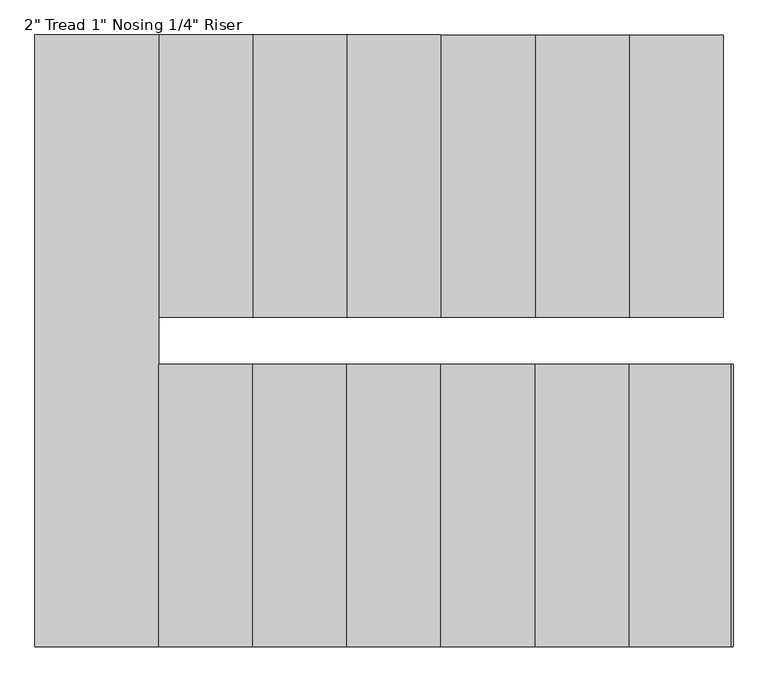
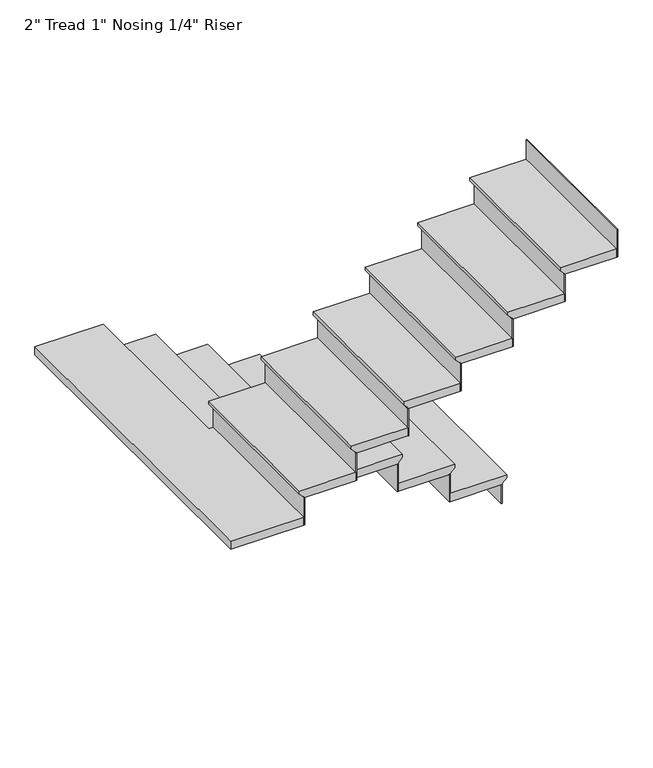
"""IFC4 building model written with IfcOpenShell, lengths in millimetres: stair flight geometry."""

from ifc_helpers import new_model, si_unit, origin, place, context, project, spatial, faceted_brep, source, transform, mapped, element, save


def stair_flight_2ee17b95(model_context):
    return source(origin(), model_context, "Body", "Brep", [
        faceted_brep([(3727.9146873, 3708.4, 3198.2833333), (3727.9146873, 3708.4, 3217.3333333), (3727.9146873, 2794.0, 3217.3333333), (3727.9146873, 2794.0, 3198.2833333), (3702.5146873, 3708.4, 3172.8833333), (3702.5146873, 2794.0, 3172.8833333), (3397.7146873, 3708.4, 3217.3333333), (3397.7146873, 2794.0, 3217.3333333), (3702.5146873, 2794.0, 3166.5333333), (3397.7146873, 2794.0, 3166.5333333), (3397.7146873, 3708.4, 3166.5333333), (3702.5146873, 3708.4, 3166.5333333)], [[[0, 1, 2, 3]], [[4, 0, 3, 5]], [[2, 1, 6, 7]], [[8, 9, 10, 11]], [[2, 7, 9, 8, 5, 3]], [[8, 11, 4, 5]], [[6, 1, 0, 4, 11, 10]], [[7, 6, 10, 9]]]),
        faceted_brep([(3702.5146873, 3708.4, 3166.5333333), (3702.5146873, 3708.4, 3048.0), (3696.1646873, 3708.4, 3048.0), (3696.1646873, 3708.4, 3166.5333333), (3702.5146873, 2794.0, 3166.5333333), (3696.1646873, 2794.0, 3166.5333333), (3696.1646873, 2794.0, 3048.0), (3702.5146873, 2794.0, 3048.0)], [[[0, 1, 2, 3]], [[4, 5, 6, 7]], [[1, 0, 4, 7]], [[2, 1, 7, 6]], [[3, 2, 6, 5]], [[0, 3, 5, 4]]]),
        faceted_brep([(3397.7146873, 3708.4, 3335.8666667), (3397.7146873, 3708.4, 3166.5333333), (3391.3646873, 3708.4, 3166.5333333), (3391.3646873, 3708.4, 3335.8666667), (3397.7146873, 2794.0, 3335.8666667), (3391.3646873, 2794.0, 3335.8666667), (3391.3646873, 2794.0, 3166.5333333), (3397.7146873, 2794.0, 3166.5333333)], [[[0, 1, 2, 3]], [[4, 5, 6, 7]], [[1, 0, 4, 7]], [[2, 1, 7, 6]], [[3, 2, 6, 5]], [[0, 3, 5, 4]]]),
        faceted_brep([(3423.1146873, 2794.0, 3386.6666667), (3423.1146873, 3708.4, 3386.6666667), (3092.9146873, 3708.4, 3386.6666667), (3092.9146873, 2794.0, 3386.6666667), (3397.7146873, 2794.0, 3335.8666667), (3092.9146873, 2794.0, 3335.8666667), (3092.9146873, 3708.4, 3335.8666667), (3397.7146873, 3708.4, 3335.8666667), (3397.7146873, 2794.0, 3342.2166667), (3423.1146873, 2794.0, 3367.6166667), (3397.7146873, 3708.4, 3342.2166667), (3423.1146873, 3708.4, 3367.6166667)], [[[0, 1, 2, 3]], [[4, 5, 6, 7]], [[0, 3, 5, 4, 8, 9]], [[4, 7, 10, 8]], [[2, 1, 11, 10, 7, 6]], [[3, 2, 6, 5]], [[11, 1, 0, 9]], [[10, 11, 9, 8]]]),
        faceted_brep([(3092.9146873, 3708.4, 3505.2), (3092.9146873, 3708.4, 3335.8666667), (3086.5646873, 3708.4, 3335.8666667), (3086.5646873, 3708.4, 3505.2), (3092.9146873, 2794.0, 3505.2), (3086.5646873, 2794.0, 3505.2), (3086.5646873, 2794.0, 3335.8666667), (3092.9146873, 2794.0, 3335.8666667)], [[[0, 1, 2, 3]], [[4, 5, 6, 7]], [[1, 0, 4, 7]], [[2, 1, 7, 6]], [[3, 2, 6, 5]], [[0, 3, 5, 4]]]),
        faceted_brep([(3118.3146873, 2794.0, 3556.0), (3118.3146873, 3708.4, 3556.0), (2788.1146873, 3708.4, 3556.0), (2788.1146873, 2794.0, 3556.0), (3092.9146873, 2794.0, 3505.2), (2788.1146873, 2794.0, 3505.2), (2788.1146873, 3708.4, 3505.2), (3092.9146873, 3708.4, 3505.2), (3092.9146873, 2794.0, 3511.55), (3118.3146873, 2794.0, 3536.95), (3092.9146873, 3708.4, 3511.55), (3118.3146873, 3708.4, 3536.95)], [[[0, 1, 2, 3]], [[4, 5, 6, 7]], [[0, 3, 5, 4, 8, 9]], [[4, 7, 10, 8]], [[2, 1, 11, 10, 7, 6]], [[3, 2, 6, 5]], [[11, 1, 0, 9]], [[10, 11, 9, 8]]]),
        faceted_brep([(2788.1146873, 3708.4, 3674.5333333), (2788.1146873, 3708.4, 3505.2), (2781.7646873, 3708.4, 3505.2), (2781.7646873, 3708.4, 3674.5333333), (2788.1146873, 2794.0, 3674.5333333), (2781.7646873, 2794.0, 3674.5333333), (2781.7646873, 2794.0, 3505.2), (2788.1146873, 2794.0, 3505.2)], [[[0, 1, 2, 3]], [[4, 5, 6, 7]], [[1, 0, 4, 7]], [[2, 1, 7, 6]], [[3, 2, 6, 5]], [[0, 3, 5, 4]]]),
        faceted_brep([(2813.5146873, 2794.0, 3725.3333333), (2813.5146873, 3708.4, 3725.3333333), (2483.3146873, 3708.4, 3725.3333333), (2483.3146873, 2794.0, 3725.3333333), (2788.1146873, 2794.0, 3674.5333333), (2483.3146873, 2794.0, 3674.5333333), (2483.3146873, 3708.4, 3674.5333333), (2788.1146873, 3708.4, 3674.5333333), (2788.1146873, 2794.0, 3680.8833333), (2813.5146873, 2794.0, 3706.2833333), (2788.1146873, 3708.4, 3680.8833333), (2813.5146873, 3708.4, 3706.2833333)], [[[0, 1, 2, 3]], [[4, 5, 6, 7]], [[0, 3, 5, 4, 8, 9]], [[4, 7, 10, 8]], [[2, 1, 11, 10, 7, 6]], [[3, 2, 6, 5]], [[11, 1, 0, 9]], [[10, 11, 9, 8]]]),
        faceted_brep([(2483.3146873, 3708.4, 3843.8666667), (2483.3146873, 3708.4, 3674.5333333), (2476.9646873, 3708.4, 3674.5333333), (2476.9646873, 3708.4, 3843.8666667), (2483.3146873, 2794.0, 3843.8666667), (2476.9646873, 2794.0, 3843.8666667), (2476.9646873, 2794.0, 3674.5333333), (2483.3146873, 2794.0, 3674.5333333)], [[[0, 1, 2, 3]], [[4, 5, 6, 7]], [[1, 0, 4, 7]], [[2, 1, 7, 6]], [[3, 2, 6, 5]], [[0, 3, 5, 4]]]),
        faceted_brep([(2508.7146873, 2794.0, 3894.6666667), (2508.7146873, 3708.4, 3894.6666667), (2178.5146873, 3708.4, 3894.6666667), (2178.5146873, 2794.0, 3894.6666667), (2483.3146873, 2794.0, 3843.8666667), (2178.5146873, 2794.0, 3843.8666667), (2178.5146873, 3708.4, 3843.8666667), (2483.3146873, 3708.4, 3843.8666667), (2483.3146873, 2794.0, 3850.2166667), (2508.7146873, 2794.0, 3875.6166667), (2483.3146873, 3708.4, 3850.2166667), (2508.7146873, 3708.4, 3875.6166667)], [[[0, 1, 2, 3]], [[4, 5, 6, 7]], [[0, 3, 5, 4, 8, 9]], [[4, 7, 10, 8]], [[2, 1, 11, 10, 7, 6]], [[3, 2, 6, 5]], [[11, 1, 0, 9]], [[10, 11, 9, 8]]]),
        faceted_brep([(2178.5146873, 3708.4, 4013.2), (2178.5146873, 3708.4, 3843.8666667), (2172.1646873, 3708.4, 3843.8666667), (2172.1646873, 3708.4, 4013.2), (2178.5146873, 2794.0, 4013.2), (2172.1646873, 2794.0, 4013.2), (2172.1646873, 2794.0, 3843.8666667), (2178.5146873, 2794.0, 3843.8666667)], [[[0, 1, 2, 3]], [[4, 5, 6, 7]], [[1, 0, 4, 7]], [[2, 1, 7, 6]], [[3, 2, 6, 5]], [[0, 3, 5, 4]]]),
        faceted_brep([(2203.9146873, 2794.0, 4064.0), (2203.9146873, 3708.4, 4064.0), (1873.7146873, 3708.4, 4064.0), (1873.7146873, 2794.0, 4064.0), (2178.5146873, 2794.0, 4013.2), (1873.7146873, 2794.0, 4013.2), (1873.7146873, 3708.4, 4013.2), (2178.5146873, 3708.4, 4013.2), (2178.5146873, 2794.0, 4019.55), (2203.9146873, 2794.0, 4044.95), (2178.5146873, 3708.4, 4019.55), (2203.9146873, 3708.4, 4044.95)], [[[0, 1, 2, 3]], [[4, 5, 6, 7]], [[0, 3, 5, 4, 8, 9]], [[4, 7, 10, 8]], [[2, 1, 11, 10, 7, 6]], [[3, 2, 6, 5]], [[11, 1, 0, 9]], [[10, 11, 9, 8]]]),
        faceted_brep([(1873.7146873, 3708.4, 4182.5333333), (1873.7146873, 3708.4, 4013.2), (1867.3646873, 3708.4, 4013.2), (1867.3646873, 3708.4, 4182.5333333), (1873.7146873, 2794.0, 4182.5333333), (1867.3646873, 2794.0, 4182.5333333), (1867.3646873, 2794.0, 4013.2), (1873.7146873, 2794.0, 4013.2)], [[[0, 1, 2, 3]], [[4, 5, 6, 7]], [[1, 0, 4, 7]], [[2, 1, 7, 6]], [[3, 2, 6, 5]], [[0, 3, 5, 4]]]),
        faceted_brep([(1924.5146873, 2641.6, 4233.3333333), (1899.1146873, 2641.6, 4233.3333333), (1899.1146873, 3708.4, 4233.3333333), (1498.6, 3708.4, 4233.3333333), (1498.6, 1727.2, 4233.3333333), (1924.5146873, 1727.2, 4233.3333333), (1899.1146873, 2641.6, 4182.5333333), (1924.5146873, 2641.6, 4182.5333333), (1924.5146873, 1727.2, 4182.5333333), (1498.6, 1727.2, 4182.5333333), (1498.6, 3708.4, 4182.5333333), (1873.7146873, 3708.4, 4182.5333333), (1873.7146873, 2794.0, 4182.5333333), (1899.1146873, 2794.0, 4182.5333333), (1899.1146873, 2794.0, 4214.2833333), (1899.1146873, 3708.4, 4214.2833333), (1873.7146873, 2794.0, 4188.8833333), (1873.7146873, 3708.4, 4188.8833333)], [[[0, 1, 2, 3, 4, 5]], [[6, 7, 8, 9, 10, 11, 12, 13]], [[1, 0, 7, 6]], [[2, 1, 6, 13, 14, 15]], [[13, 12, 16, 14]], [[12, 11, 17, 16]], [[3, 2, 15, 17, 11, 10]], [[4, 3, 10, 9]], [[5, 4, 9, 8]], [[0, 5, 8, 7]], [[17, 15, 14, 16]]]),
        faceted_brep([(1924.5146873, 1727.2, 4351.8666667), (1924.5146873, 1727.2, 4182.5333333), (1930.8646873, 1727.2, 4182.5333333), (1930.8646873, 1727.2, 4351.8666667), (1924.5146873, 2641.6, 4351.8666667), (1930.8646873, 2641.6, 4351.8666667), (1930.8646873, 2641.6, 4182.5333333), (1924.5146873, 2641.6, 4182.5333333)], [[[0, 1, 2, 3]], [[4, 5, 6, 7]], [[1, 0, 4, 7]], [[2, 1, 7, 6]], [[3, 2, 6, 5]], [[0, 3, 5, 4]]]),
        faceted_brep([(1899.1146873, 2641.6, 4402.6666667), (1899.1146873, 1727.2, 4402.6666667), (2229.3146873, 1727.2, 4402.6666667), (2229.3146873, 2641.6, 4402.6666667), (1924.5146873, 2641.6, 4351.8666667), (2229.3146873, 2641.6, 4351.8666667), (2229.3146873, 1727.2, 4351.8666667), (1924.5146873, 1727.2, 4351.8666667), (1924.5146873, 2641.6, 4358.2166667), (1899.1146873, 2641.6, 4383.6166667), (1924.5146873, 1727.2, 4358.2166667), (1899.1146873, 1727.2, 4383.6166667)], [[[0, 1, 2, 3]], [[4, 5, 6, 7]], [[0, 3, 5, 4, 8, 9]], [[4, 7, 10, 8]], [[2, 1, 11, 10, 7, 6]], [[3, 2, 6, 5]], [[11, 1, 0, 9]], [[10, 11, 9, 8]]]),
        faceted_brep([(2229.3146873, 1727.2, 4521.2), (2229.3146873, 1727.2, 4351.8666667), (2235.6646873, 1727.2, 4351.8666667), (2235.6646873, 1727.2, 4521.2), (2229.3146873, 2641.6, 4521.2), (2235.6646873, 2641.6, 4521.2), (2235.6646873, 2641.6, 4351.8666667), (2229.3146873, 2641.6, 4351.8666667)], [[[0, 1, 2, 3]], [[4, 5, 6, 7]], [[1, 0, 4, 7]], [[2, 1, 7, 6]], [[3, 2, 6, 5]], [[0, 3, 5, 4]]]),
        faceted_brep([(2203.9146873, 2641.6, 4572.0), (2203.9146873, 1727.2, 4572.0), (2534.1146873, 1727.2, 4572.0), (2534.1146873, 2641.6, 4572.0), (2229.3146873, 2641.6, 4521.2), (2534.1146873, 2641.6, 4521.2), (2534.1146873, 1727.2, 4521.2), (2229.3146873, 1727.2, 4521.2), (2229.3146873, 2641.6, 4527.55), (2203.9146873, 2641.6, 4552.95), (2229.3146873, 1727.2, 4527.55), (2203.9146873, 1727.2, 4552.95)], [[[0, 1, 2, 3]], [[4, 5, 6, 7]], [[0, 3, 5, 4, 8, 9]], [[4, 7, 10, 8]], [[2, 1, 11, 10, 7, 6]], [[3, 2, 6, 5]], [[11, 1, 0, 9]], [[10, 11, 9, 8]]]),
        faceted_brep([(2534.1146873, 1727.2, 4690.5333333), (2534.1146873, 1727.2, 4521.2), (2540.4646873, 1727.2, 4521.2), (2540.4646873, 1727.2, 4690.5333333), (2534.1146873, 2641.6, 4690.5333333), (2540.4646873, 2641.6, 4690.5333333), (2540.4646873, 2641.6, 4521.2), (2534.1146873, 2641.6, 4521.2)], [[[0, 1, 2, 3]], [[4, 5, 6, 7]], [[1, 0, 4, 7]], [[2, 1, 7, 6]], [[3, 2, 6, 5]], [[0, 3, 5, 4]]]),
        faceted_brep([(2508.7146873, 2641.6, 4741.3333333), (2508.7146873, 1727.2, 4741.3333333), (2838.9146873, 1727.2, 4741.3333333), (2838.9146873, 2641.6, 4741.3333333), (2534.1146873, 2641.6, 4690.5333333), (2838.9146873, 2641.6, 4690.5333333), (2838.9146873, 1727.2, 4690.5333333), (2534.1146873, 1727.2, 4690.5333333), (2534.1146873, 2641.6, 4696.8833333), (2508.7146873, 2641.6, 4722.2833333), (2534.1146873, 1727.2, 4696.8833333), (2508.7146873, 1727.2, 4722.2833333)], [[[0, 1, 2, 3]], [[4, 5, 6, 7]], [[0, 3, 5, 4, 8, 9]], [[4, 7, 10, 8]], [[2, 1, 11, 10, 7, 6]], [[3, 2, 6, 5]], [[11, 1, 0, 9]], [[10, 11, 9, 8]]]),
        faceted_brep([(2838.9146873, 1727.2, 4859.8666667), (2838.9146873, 1727.2, 4690.5333333), (2845.2646873, 1727.2, 4690.5333333), (2845.2646873, 1727.2, 4859.8666667), (2838.9146873, 2641.6, 4859.8666667), (2845.2646873, 2641.6, 4859.8666667), (2845.2646873, 2641.6, 4690.5333333), (2838.9146873, 2641.6, 4690.5333333)], [[[0, 1, 2, 3]], [[4, 5, 6, 7]], [[1, 0, 4, 7]], [[2, 1, 7, 6]], [[3, 2, 6, 5]], [[0, 3, 5, 4]]]),
        faceted_brep([(2813.5146873, 2641.6, 4910.6666667), (2813.5146873, 1727.2, 4910.6666667), (3143.7146873, 1727.2, 4910.6666667), (3143.7146873, 2641.6, 4910.6666667), (2838.9146873, 2641.6, 4859.8666667), (3143.7146873, 2641.6, 4859.8666667), (3143.7146873, 1727.2, 4859.8666667), (2838.9146873, 1727.2, 4859.8666667), (2838.9146873, 2641.6, 4866.2166667), (2813.5146873, 2641.6, 4891.6166667), (2838.9146873, 1727.2, 4866.2166667), (2813.5146873, 1727.2, 4891.6166667)], [[[0, 1, 2, 3]], [[4, 5, 6, 7]], [[0, 3, 5, 4, 8, 9]], [[4, 7, 10, 8]], [[2, 1, 11, 10, 7, 6]], [[3, 2, 6, 5]], [[11, 1, 0, 9]], [[10, 11, 9, 8]]]),
        faceted_brep([(3143.7146873, 1727.2, 5029.2), (3143.7146873, 1727.2, 4859.8666667), (3150.0646873, 1727.2, 4859.8666667), (3150.0646873, 1727.2, 5029.2), (3143.7146873, 2641.6, 5029.2), (3150.0646873, 2641.6, 5029.2), (3150.0646873, 2641.6, 4859.8666667), (3143.7146873, 2641.6, 4859.8666667)], [[[0, 1, 2, 3]], [[4, 5, 6, 7]], [[1, 0, 4, 7]], [[2, 1, 7, 6]], [[3, 2, 6, 5]], [[0, 3, 5, 4]]]),
        faceted_brep([(3118.3146873, 2641.6, 5080.0), (3118.3146873, 1727.2, 5080.0), (3448.5146873, 1727.2, 5080.0), (3448.5146873, 2641.6, 5080.0), (3143.7146873, 2641.6, 5029.2), (3448.5146873, 2641.6, 5029.2), (3448.5146873, 1727.2, 5029.2), (3143.7146873, 1727.2, 5029.2), (3143.7146873, 2641.6, 5035.55), (3118.3146873, 2641.6, 5060.95), (3143.7146873, 1727.2, 5035.55), (3118.3146873, 1727.2, 5060.95)], [[[0, 1, 2, 3]], [[4, 5, 6, 7]], [[0, 3, 5, 4, 8, 9]], [[4, 7, 10, 8]], [[2, 1, 11, 10, 7, 6]], [[3, 2, 6, 5]], [[11, 1, 0, 9]], [[10, 11, 9, 8]]]),
        faceted_brep([(3448.5146873, 1727.2, 5198.5333333), (3448.5146873, 1727.2, 5029.2), (3454.8646873, 1727.2, 5029.2), (3454.8646873, 1727.2, 5198.5333333), (3448.5146873, 2641.6, 5198.5333333), (3454.8646873, 2641.6, 5198.5333333), (3454.8646873, 2641.6, 5029.2), (3448.5146873, 2641.6, 5029.2)], [[[0, 1, 2, 3]], [[4, 5, 6, 7]], [[1, 0, 4, 7]], [[2, 1, 7, 6]], [[3, 2, 6, 5]], [[0, 3, 5, 4]]]),
        faceted_brep([(3753.3146873, 1727.2, 5367.8666667), (3753.3146873, 1727.2, 5198.5333333), (3759.6646873, 1727.2, 5198.5333333), (3759.6646873, 1727.2, 5367.8666667), (3753.3146873, 2641.6, 5367.8666667), (3759.6646873, 2641.6, 5367.8666667), (3759.6646873, 2641.6, 5198.5333333), (3753.3146873, 2641.6, 5198.5333333)], [[[0, 1, 2, 3]], [[4, 5, 6, 7]], [[1, 0, 4, 7]], [[2, 1, 7, 6]], [[3, 2, 6, 5]], [[0, 3, 5, 4]]]),
        faceted_brep([(3423.1146873, 2641.6, 5249.3333333), (3423.1146873, 1727.2, 5249.3333333), (3753.3146873, 1727.2, 5249.3333333), (3753.3146873, 2641.6, 5249.3333333), (3448.5146873, 2641.6, 5198.5333333), (3753.3146873, 2641.6, 5198.5333333), (3753.3146873, 1727.2, 5198.5333333), (3448.5146873, 1727.2, 5198.5333333), (3448.5146873, 2641.6, 5204.8833333), (3423.1146873, 2641.6, 5230.2833333), (3448.5146873, 1727.2, 5204.8833333), (3423.1146873, 1727.2, 5230.2833333)], [[[0, 1, 2, 3]], [[4, 5, 6, 7]], [[0, 3, 5, 4, 8, 9]], [[4, 7, 10, 8]], [[2, 1, 11, 10, 7, 6]], [[3, 2, 6, 5]], [[11, 1, 0, 9]], [[10, 11, 9, 8]]]),
    ])


if __name__ == "__main__":
    model = new_model("IFC4")
    model_context = context("Model", 3, world=origin())
    ifc_project = project(units=[si_unit("LENGTHUNIT", "METRE", prefix="MILLI")], contexts=[model_context])
    site = spatial("IfcSite", under=ifc_project)
    building = spatial("IfcBuilding", under=site)
    placement = place(None, origin())
    stair_flight_shape = stair_flight_2ee17b95(model_context)
    element("IfcStairFlight", 1, ObjectType="2\" Tread 1\" Nosing 1/4\" Riser", at=placement, inside=building, context=model_context, shape_type="MappedRepresentation", body=[
        mapped(stair_flight_shape, transform((0.0, 0.0, 0.0), x_axis=(1.0, 0.0, 0.0), y_axis=(0.0, 1.0, 0.0), z_axis=(0.0, 0.0, 1.0))),
    ])
    save(model, "model.ifc")
